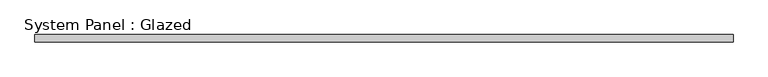
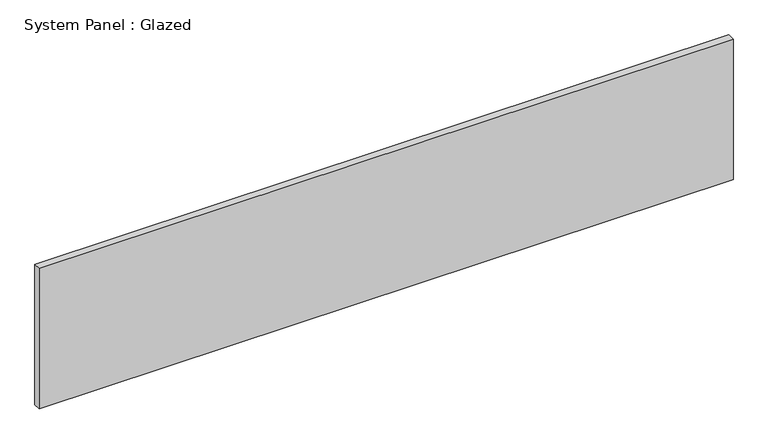
"""IFC4 building model written with IfcOpenShell, lengths in millimetres: plate geometry, System Panel : Glazed."""

from ifc_helpers import new_model, si_unit, origin, origin_with_axes, place, context, project, spatial, polyline, outline, extrude, source, transform, mapped, element, save


def system_panel_glazed_c8d94a63(model_context):
    return source(origin(), model_context, "Body", "SweptSolid", [
        extrude(outline(polyline([(1216.025, 19.05), (-1216.025, 19.05), (-1216.025, 44.45), (1216.025, 44.45), (1216.025, 19.05)])), origin_with_axes(), (0.0, 0.0, 1.0), 520.7173759),
    ])


if __name__ == "__main__":
    model = new_model("IFC4")
    model_context = context("Model", 3, world=origin())
    ifc_project = project(units=[si_unit("LENGTHUNIT", "METRE", prefix="MILLI")], contexts=[model_context])
    site = spatial("IfcSite", under=ifc_project)
    building = spatial("IfcBuilding", under=site)
    placement = place(None, origin())
    system_panel_glazed_shape = system_panel_glazed_c8d94a63(model_context)
    element("IfcPlate", 1, ObjectType="System Panel : Glazed", at=placement, inside=building, context=model_context, shape_type="MappedRepresentation", body=[
        mapped(system_panel_glazed_shape, transform((0.0, 0.0, 0.0), x_axis=(1.0, 0.0, 0.0), y_axis=(0.0, 1.0, 0.0), z_axis=(0.0, 0.0, 1.0))),
    ])
    save(model, "model.ifc")

# Revit data of these elements
# Type "System Panel : Glazed"
#   Construction Type Id = "GSP4R"
#   Analytic Construction = "1/8 in Pilkington single glazing"
#   Visual Light Transmittance = 0.9
#   Solar Heat Gain Coefficient = 0.86
#   Heat Transfer Coefficient (U) = 1.18115 BTU/(h·ft²·°F)
#   Define Thermal Properties by = 1
# Element 1 (IfcPlate, "System Panel : Glazed")
#   Materials on its faces: "Glass"
# Materials
#   "Glass": class "Glass", colour RGB 0 128 192, transparency 0.75, Description = "Soda Lime Glass", Cost = 0
